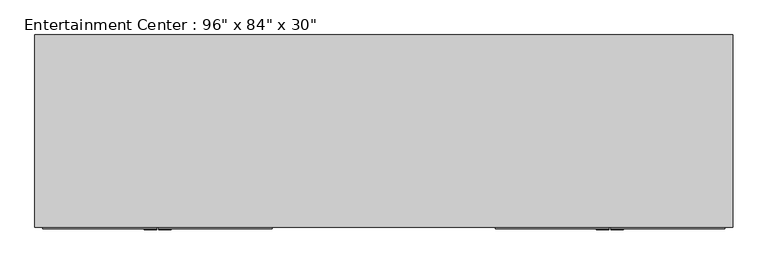
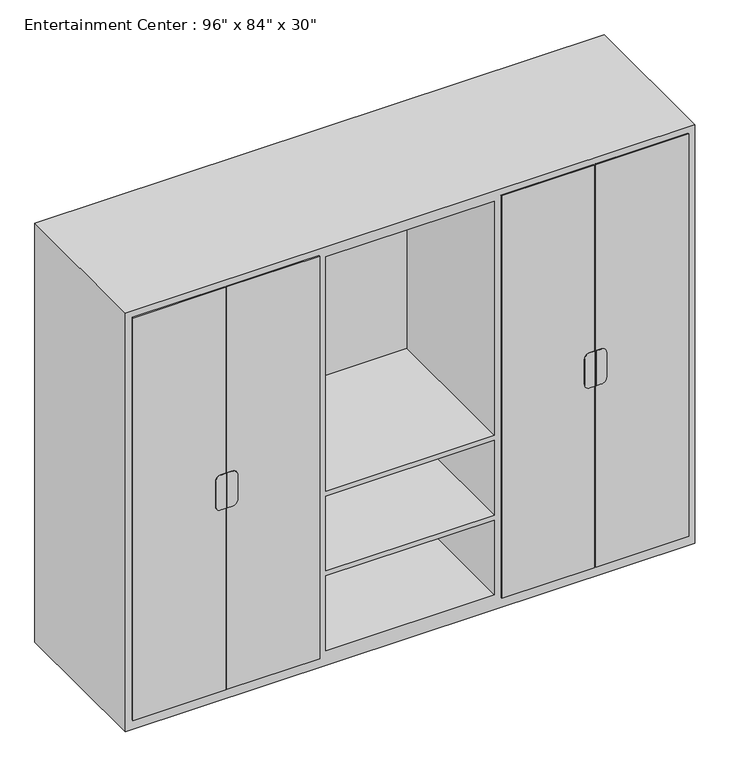
"""IFC4 building model written with IfcOpenShell, lengths in millimetres: furniture geometry."""

from ifc_helpers import new_model, si_unit, point, frame, frame_2d, origin, place, context, project, spatial, polyline, circle_curve, trimmed, segment, composite_curve, outline, extrude, faceted_brep, source, transform, mapped, element, save


def furniture_1f19b6cd(model_context):
    return source(origin(), model_context, "Body", "SolidModel", [
        extrude(outline(polyline([(-1339.85, -781.05), (-892.175, -781.05), (-892.175, -787.4), (-1339.85, -787.4), (-1339.85, -781.05)])), frame((0.0, 0.0, 50.8), z_axis=(0.0, 0.0, 1.0), x_axis=(1.0, 0.0, 0.0)), (0.0, 0.0, 1.0), 2051.05),
        extrude(outline(polyline([(-885.825, -781.05), (-438.15, -781.05), (-438.15, -787.4), (-885.825, -787.4), (-885.825, -781.05)])), frame((0.0, 0.0, 50.8), z_axis=(0.0, 0.0, 1.0), x_axis=(1.0, 0.0, 0.0)), (0.0, 0.0, 1.0), 2051.05),
        extrude(outline(polyline([(892.175, -781.05), (1339.85, -781.05), (1339.85, -787.4), (892.175, -787.4), (892.175, -781.05)])), frame((0.0, 0.0, 50.8), z_axis=(0.0, 0.0, 1.0), x_axis=(1.0, 0.0, 0.0)), (0.0, 0.0, 1.0), 2051.05),
        extrude(outline(polyline([(438.15, -781.05), (885.825, -781.05), (885.825, -787.4), (438.15, -787.4), (438.15, -781.05)])), frame((0.0, 0.0, 50.8), z_axis=(0.0, 0.0, 1.0), x_axis=(1.0, 0.0, 0.0)), (0.0, 0.0, 1.0), 2051.05),
        extrude(outline(composite_curve([segment(polyline([(1155.7, -861.5986452), (1155.7, -885.825), (977.9, -885.825), (977.9, -861.5986452)]), True, "CONTINUOUS"), segment(trimmed(circle_curve(frame_2d((1003.3, -861.5986452)), 25.4), [point((977.9, -861.5986452))], [point((1003.3, -836.1986452))], False, "CARTESIAN"), True, "CONTINUOUS"), segment(polyline([(1003.3, -836.1986452), (1130.3, -836.1986452)]), True, "CONTINUOUS"), segment(trimmed(circle_curve(frame_2d((1130.3, -861.5986452)), 25.4), [point((1130.3, -836.1986452))], [point((1155.7, -861.5986452))], False, "CARTESIAN"), True, "CONTINUOUS")], self_intersect=False)), frame((0.0, -790.575, 0.0), z_axis=(0.0, 1.0, 0.0), x_axis=(0.0, 0.0, 1.0)), (0.0, 0.0, 1.0), 3.175),
        extrude(outline(composite_curve([segment(trimmed(circle_curve(frame_2d((1130.3, -916.78125)), 25.4), [point((1155.7, -916.78125))], [point((1130.3, -942.18125))], False, "CARTESIAN"), True, "CONTINUOUS"), segment(polyline([(1130.3, -942.18125), (1003.3, -942.18125)]), True, "CONTINUOUS"), segment(trimmed(circle_curve(frame_2d((1003.3, -916.78125)), 25.4), [point((1003.3, -942.18125))], [point((977.9, -916.78125))], False, "CARTESIAN"), True, "CONTINUOUS"), segment(polyline([(977.9, -916.78125), (977.9, -892.175), (1155.7, -892.175), (1155.7, -916.78125)]), True, "CONTINUOUS")], self_intersect=False)), frame((0.0, -790.575, 0.0), z_axis=(0.0, 1.0, 0.0), x_axis=(0.0, 0.0, 1.0)), (0.0, 0.0, 1.0), 3.175),
        extrude(outline(composite_curve([segment(trimmed(circle_curve(frame_2d((1130.3, 861.5986452)), 25.4), [point((1155.7, 861.5986452))], [point((1130.3, 836.1986452))], False, "CARTESIAN"), True, "CONTINUOUS"), segment(polyline([(1130.3, 836.1986452), (1003.3, 836.1986452)]), True, "CONTINUOUS"), segment(trimmed(circle_curve(frame_2d((1003.3, 861.5986452)), 25.4), [point((1003.3, 836.1986452))], [point((977.9, 861.5986452))], False, "CARTESIAN"), True, "CONTINUOUS"), segment(polyline([(977.9, 861.5986452), (977.9, 885.825), (1155.7, 885.825), (1155.7, 861.5986452)]), True, "CONTINUOUS")], self_intersect=False)), frame((0.0, -790.575, 0.0), z_axis=(0.0, 1.0, 0.0), x_axis=(0.0, 0.0, 1.0)), (0.0, 0.0, 1.0), 3.175),
        extrude(outline(composite_curve([segment(polyline([(1155.7, 916.78125), (1155.7, 892.175), (977.9, 892.175), (977.9, 916.78125)]), True, "CONTINUOUS"), segment(trimmed(circle_curve(frame_2d((1003.3, 916.78125)), 25.4), [point((977.9, 916.78125))], [point((1003.3, 942.18125))], False, "CARTESIAN"), True, "CONTINUOUS"), segment(polyline([(1003.3, 942.18125), (1130.3, 942.18125)]), True, "CONTINUOUS"), segment(trimmed(circle_curve(frame_2d((1130.3, 916.78125)), 25.4), [point((1130.3, 942.18125))], [point((1155.7, 916.78125))], False, "CARTESIAN"), True, "CONTINUOUS")], self_intersect=False)), frame((0.0, -790.575, 0.0), z_axis=(0.0, 1.0, 0.0), x_axis=(0.0, 0.0, 1.0)), (0.0, 0.0, 1.0), 3.175),
        faceted_brep([(1371.6, -781.05, 0.0), (1371.6, -781.05, 2133.6), (-1371.6, -781.05, 2133.6), (-1371.6, -781.05, 0.0), (-457.2, -781.05, 2082.8), (-457.2, -781.05, 1612.9), (-1320.8, -781.05, 1612.9), (-1320.8, -781.05, 2082.8), (-457.2, -781.05, 76.2), (-1320.8, -781.05, 76.2), (-1320.8, -781.05, 520.7), (-457.2, -781.05, 520.7), (1320.8, -781.05, 1612.9), (457.2, -781.05, 1612.9), (457.2, -781.05, 2082.8), (1320.8, -781.05, 2082.8), (-406.4, -781.05, 889.0), (-406.4, -781.05, 2082.8), (406.4, -781.05, 2082.8), (406.4, -781.05, 889.0), (406.4, -781.05, 76.2), (-406.4, -781.05, 76.2), (-406.4, -781.05, 457.2), (406.4, -781.05, 457.2), (1320.8, -781.05, 76.2), (457.2, -781.05, 76.2), (457.2, -781.05, 520.7), (1320.8, -781.05, 520.7), (-1320.8, -781.05, 546.1), (-1320.8, -781.05, 1054.1), (-457.2, -781.05, 1054.1), (-457.2, -781.05, 546.1), (-457.2, -781.05, 1587.5), (-457.2, -781.05, 1079.5), (-1320.8, -781.05, 1079.5), (-1320.8, -781.05, 1587.5), (457.2, -781.05, 1587.5), (1320.8, -781.05, 1587.5), (1320.8, -781.05, 1079.5), (457.2, -781.05, 1079.5), (457.2, -781.05, 1054.1), (1320.8, -781.05, 1054.1), (1320.8, -781.05, 546.1), (457.2, -781.05, 546.1), (406.4, -781.05, 482.6), (-406.4, -781.05, 482.6), (-406.4, -781.05, 863.6), (406.4, -781.05, 863.6), (1371.6, -25.4, 0.0), (-1371.6, -25.4, 0.0), (-1371.6, -25.4, 2133.6), (1371.6, -25.4, 2133.6), (-457.2, -50.8, 2082.8), (-457.2, -50.8, 1612.9), (-1320.8, -50.8, 1612.9), (-1320.8, -50.8, 2082.8), (-457.2, -50.8, 76.2), (-1320.8, -50.8, 76.2), (-1320.8, -50.8, 520.7), (-457.2, -50.8, 520.7), (1320.8, -50.8, 1612.9), (457.2, -50.8, 1612.9), (457.2, -50.8, 2082.8), (1320.8, -50.8, 2082.8), (-406.4, -50.8, 889.0), (-406.4, -50.8, 2082.8), (406.4, -50.8, 2082.8), (406.4, -50.8, 889.0), (406.4, -50.8, 76.2), (-406.4, -50.8, 76.2), (-406.4, -50.8, 457.2), (406.4, -50.8, 457.2), (1320.8, -50.8, 76.2), (457.2, -50.8, 76.2), (457.2, -50.8, 520.7), (1320.8, -50.8, 520.7), (-1320.8, -50.8, 546.1), (-1320.8, -50.8, 1054.1), (-457.2, -50.8, 1054.1), (-457.2, -50.8, 546.1), (-457.2, -50.8, 1587.5), (-457.2, -50.8, 1079.5), (-1320.8, -50.8, 1079.5), (-1320.8, -50.8, 1587.5), (457.2, -50.8, 1587.5), (1320.8, -50.8, 1587.5), (1320.8, -50.8, 1079.5), (457.2, -50.8, 1079.5), (457.2, -50.8, 1054.1), (1320.8, -50.8, 1054.1), (1320.8, -50.8, 546.1), (457.2, -50.8, 546.1), (406.4, -50.8, 482.6), (-406.4, -50.8, 482.6), (-406.4, -50.8, 863.6), (406.4, -50.8, 863.6)], [[[0, 1, 2, 3], [4, 5, 6, 7], [8, 9, 10, 11], [12, 13, 14, 15], [16, 17, 18, 19], [20, 21, 22, 23], [24, 25, 26, 27], [28, 29, 30, 31], [32, 33, 34, 35], [36, 37, 38, 39], [40, 41, 42, 43], [44, 45, 46, 47]], [[48, 49, 50, 51]], [[1, 0, 48, 51]], [[2, 1, 51, 50]], [[3, 2, 50, 49]], [[0, 3, 49, 48]], [[5, 4, 52, 53]], [[6, 5, 53, 54]], [[7, 6, 54, 55]], [[4, 7, 55, 52]], [[9, 8, 56, 57]], [[10, 9, 57, 58]], [[11, 10, 58, 59]], [[8, 11, 59, 56]], [[13, 12, 60, 61]], [[14, 13, 61, 62]], [[15, 14, 62, 63]], [[12, 15, 63, 60]], [[17, 16, 64, 65]], [[18, 17, 65, 66]], [[19, 18, 66, 67]], [[16, 19, 67, 64]], [[21, 20, 68, 69]], [[22, 21, 69, 70]], [[23, 22, 70, 71]], [[20, 23, 71, 68]], [[25, 24, 72, 73]], [[26, 25, 73, 74]], [[27, 26, 74, 75]], [[24, 27, 75, 72]], [[29, 28, 76, 77]], [[30, 29, 77, 78]], [[31, 30, 78, 79]], [[28, 31, 79, 76]], [[33, 32, 80, 81]], [[34, 33, 81, 82]], [[35, 34, 82, 83]], [[32, 35, 83, 80]], [[37, 36, 84, 85]], [[38, 37, 85, 86]], [[39, 38, 86, 87]], [[36, 39, 87, 84]], [[41, 40, 88, 89]], [[42, 41, 89, 90]], [[43, 42, 90, 91]], [[40, 43, 91, 88]], [[45, 44, 92, 93]], [[46, 45, 93, 94]], [[47, 46, 94, 95]], [[44, 47, 95, 92]], [[53, 52, 55, 54]], [[57, 56, 59, 58]], [[61, 60, 63, 62]], [[65, 64, 67, 66]], [[69, 68, 71, 70]], [[73, 72, 75, 74]], [[77, 76, 79, 78]], [[81, 80, 83, 82]], [[85, 84, 87, 86]], [[89, 88, 91, 90]], [[93, 92, 95, 94]]]),
    ])


if __name__ == "__main__":
    model = new_model("IFC4")
    model_context = context("Model", 3, world=origin())
    ifc_project = project(units=[si_unit("LENGTHUNIT", "METRE", prefix="MILLI")], contexts=[model_context])
    site = spatial("IfcSite", under=ifc_project)
    building = spatial("IfcBuilding", under=site)
    placement = place(None, origin())
    furniture_shape = furniture_1f19b6cd(model_context)
    element("IfcFurniture", 1, ObjectType="Entertainment Center : 96\" x 84\" x 30\"", at=placement, inside=building, context=model_context, shape_type="MappedRepresentation", body=[
        mapped(furniture_shape, transform((0.0, 0.0, 0.0), x_axis=(1.0, 0.0, 0.0), y_axis=(0.0, 1.0, 0.0), z_axis=(0.0, 0.0, 1.0))),
    ])
    save(model, "model.ifc")

# Revit data of these elements
# Type "Entertainment Center : 96\" x 84\" x 30\""
#   Assembly Code = "E2020200"
#   Center Width = 2' - 8"
#   Depth = 2' - 6"
#   Height = 7' - 0"
#   Width = 9' - 0"
#   Material = Laminate, Ivory, Matte
#   Default Elevation = 0
# Element 1 (IfcFurniture, "Entertainment Center : 96\" x 84\" x 30\"")
#   Materials on its faces: "Laminate, Ivory, Matte", "Steel, Chrome Plated", "Glass - Clear, Grey"
# Materials
#   "Laminate, Ivory, Matte": class "Plastic", colour RGB 247 247 239, transparency 0, Description = "Plastic Laminate - Ivory, Matte", Cost = 0
#   "Steel, Chrome Plated": class "Metal", colour RGB 17 17 17, transparency 0, Description = "Chromiuim plated steel", Cost = 0
#   "Glass - Clear, Grey": class "Glass", colour RGB 252 255 255, transparency 0.64
